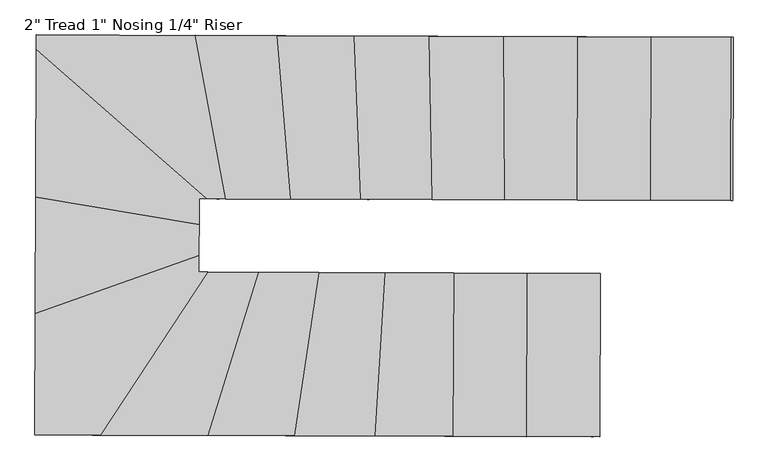
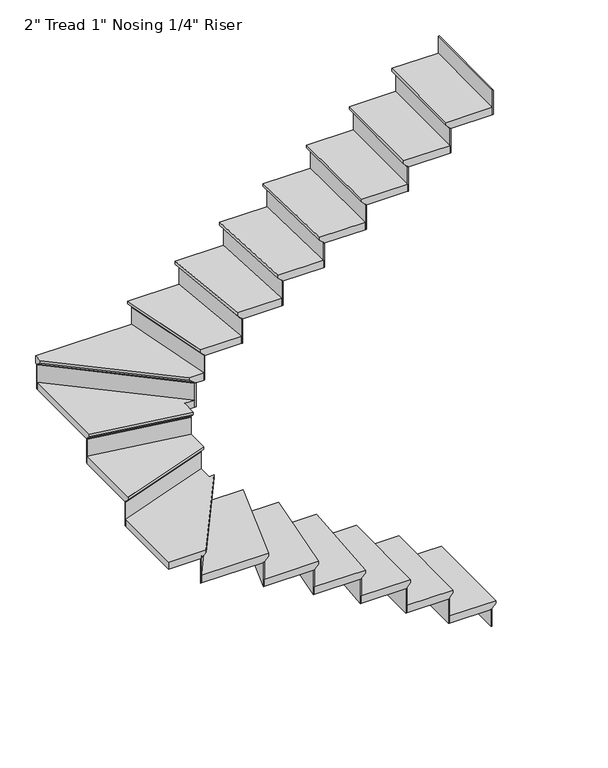
"""IFC4 building model written with IfcOpenShell, lengths in millimetres: stair flight geometry."""

from ifc_helpers import new_model, si_unit, origin, place, context, project, spatial, faceted_brep, source, transform, mapped, element, save


def stair_flight_f5e35143(model_context):
    return source(origin(), model_context, "Body", "Brep", [
        faceted_brep([(-2339.9228929, -4204.0248458, 6551.0833333), (-2339.9228929, -4204.0248458, 6570.1333333), (-2342.0274141, -4826.0015756, 6570.1333333), (-2342.0274141, -4826.0015756, 6551.0833333), (-2365.3227475, -4203.9389029, 6525.6833333), (-2367.4272687, -4825.9156326, 6525.6833333), (-2644.7211481, -4202.9935301, 6570.1333333), (-2646.8256693, -4824.9702599, 6570.1333333), (-2367.4272687, -4825.9156326, 6519.3333333), (-2646.8256693, -4824.9702599, 6519.3333333), (-2644.7211481, -4202.9935301, 6519.3333333), (-2365.3227475, -4203.9389029, 6519.3333333)], [[[0, 1, 2, 3]], [[4, 0, 3, 5]], [[2, 1, 6, 7]], [[8, 9, 10, 11]], [[2, 7, 9, 8, 5, 3]], [[8, 11, 4, 5]], [[6, 1, 0, 4, 11, 10]], [[7, 6, 10, 9]]]),
        faceted_brep([(-2365.3227475, -4203.9389029, 6519.3333333), (-2365.3227475, -4203.9389029, 6400.8), (-2371.6727112, -4203.9174171, 6400.8), (-2371.6727112, -4203.9174171, 6519.3333333), (-2367.4272687, -4825.9156326, 6519.3333333), (-2373.7772323, -4825.8941469, 6519.3333333), (-2373.7772323, -4825.8941469, 6400.8), (-2367.4272687, -4825.9156326, 6400.8)], [[[0, 1, 2, 3]], [[4, 5, 6, 7]], [[1, 0, 4, 7]], [[2, 1, 7, 6]], [[3, 2, 6, 5]], [[0, 3, 5, 4]]]),
        faceted_brep([(-2644.7211481, -4202.9935301, 6688.6666667), (-2644.7211481, -4202.9935301, 6519.3333333), (-2651.0711118, -4202.9720444, 6519.3333333), (-2651.0711118, -4202.9720444, 6688.6666667), (-2646.8256693, -4824.9702599, 6688.6666667), (-2653.175633, -4824.9487741, 6688.6666667), (-2653.175633, -4824.9487741, 6519.3333333), (-2646.8256693, -4824.9702599, 6519.3333333)], [[[0, 1, 2, 3]], [[4, 5, 6, 7]], [[1, 0, 4, 7]], [[2, 1, 7, 6]], [[3, 2, 6, 5]], [[0, 3, 5, 4]]]),
        faceted_brep([(-2621.4258147, -4825.0562028, 6739.4666667), (-2619.3212935, -4203.0794731, 6739.4666667), (-2924.1195488, -4202.0481574, 6739.4666667), (-2926.2240699, -4824.0248871, 6739.4666667), (-2646.8256693, -4824.9702599, 6688.6666667), (-2926.2240699, -4824.0248871, 6688.6666667), (-2924.1195488, -4202.0481574, 6688.6666667), (-2644.7211481, -4202.9935301, 6688.6666667), (-2646.8256693, -4824.9702599, 6695.0166667), (-2621.4258147, -4825.0562028, 6720.4166667), (-2644.7211481, -4202.9935301, 6695.0166667), (-2619.3212935, -4203.0794731, 6720.4166667)], [[[0, 1, 2, 3]], [[4, 5, 6, 7]], [[0, 3, 5, 4, 8, 9]], [[4, 7, 10, 8]], [[2, 1, 11, 10, 7, 6]], [[3, 2, 6, 5]], [[11, 1, 0, 9]], [[10, 11, 9, 8]]]),
        faceted_brep([(-2924.1195488, -4202.0481574, 6858.0), (-2924.1195488, -4202.0481574, 6688.6666667), (-2930.4695124, -4202.0266716, 6688.6666667), (-2930.4695124, -4202.0266716, 6858.0), (-2926.2240699, -4824.0248871, 6858.0), (-2932.5740336, -4824.0034014, 6858.0), (-2932.5740336, -4824.0034014, 6688.6666667), (-2926.2240699, -4824.0248871, 6688.6666667)], [[[0, 1, 2, 3]], [[4, 5, 6, 7]], [[1, 0, 4, 7]], [[2, 1, 7, 6]], [[3, 2, 6, 5]], [[0, 3, 5, 4]]]),
        faceted_brep([(-2900.8242153, -4824.1108301, 6908.8), (-2898.7196941, -4202.1341003, 6908.8), (-3185.4282049, -4201.1639931, 6908.8), (-3223.7984946, -4823.0180139, 6908.8), (-2926.2240699, -4824.0248871, 6858.0), (-3223.7984946, -4823.0180139, 6858.0), (-3185.4282049, -4201.1639931, 6858.0), (-2924.1195488, -4202.0481574, 6858.0), (-2926.2240699, -4824.0248871, 6864.35), (-2900.8242153, -4824.1108301, 6889.75), (-2924.1195488, -4202.0481574, 6864.35), (-2898.7196941, -4202.1341003, 6889.75)], [[[0, 1, 2, 3]], [[4, 5, 6, 7]], [[0, 3, 5, 4, 8, 9]], [[4, 7, 10, 8]], [[2, 1, 11, 10, 7, 6]], [[3, 2, 6, 5]], [[11, 1, 0, 9]], [[10, 11, 9, 8]]]),
        faceted_brep([(-3185.4282049, -4201.1639931, 7027.3333333), (-3185.4282049, -4201.1639931, 6858.0), (-3191.7889535, -4201.1424708, 6858.0), (-3191.7889535, -4201.1424708, 7027.3333333), (-3223.7984946, -4823.0180139, 7027.3333333), (-3230.1592432, -4822.9964917, 7027.3333333), (-3230.1592432, -4822.9964917, 6858.0), (-3223.7984946, -4823.0180139, 6858.0)], [[[0, 1, 2, 3]], [[4, 5, 6, 7]], [[1, 0, 4, 7]], [[2, 1, 7, 6]], [[3, 2, 6, 5]], [[0, 3, 5, 4]]]),
        faceted_brep([(-3198.3555003, -4823.1041029, 7078.1333333), (-3159.9852105, -4201.250082, 7078.1333333), (-3437.1491731, -4200.3122697, 7078.1333333), (-3531.3418182, -4821.97741, 7078.1333333), (-3223.7984946, -4823.0180139, 7027.3333333), (-3531.3418182, -4821.97741, 7027.3333333), (-3437.1491731, -4200.3122697, 7027.3333333), (-3185.4282049, -4201.1639931, 7027.3333333), (-3223.7984946, -4823.0180139, 7033.6833333), (-3198.3555003, -4823.1041029, 7059.0833333), (-3185.4282049, -4201.1639931, 7033.6833333), (-3159.9852105, -4201.250082, 7059.0833333)], [[[0, 1, 2, 3]], [[4, 5, 6, 7]], [[0, 3, 5, 4, 8, 9]], [[4, 7, 10, 8]], [[2, 1, 11, 10, 7, 6]], [[3, 2, 6, 5]], [[11, 1, 0, 9]], [[10, 11, 9, 8]]]),
        faceted_brep([(-3437.1491731, -4200.3122697, 7196.6666667), (-3437.1491731, -4200.3122697, 7027.3333333), (-3443.568358, -4200.2905498, 7027.3333333), (-3443.568358, -4200.2905498, 7196.6666667), (-3531.3418182, -4821.97741, 7196.6666667), (-3537.7610031, -4821.95569, 7196.6666667), (-3537.7610031, -4821.95569, 7027.3333333), (-3531.3418182, -4821.97741, 7027.3333333)], [[[0, 1, 2, 3]], [[4, 5, 6, 7]], [[1, 0, 4, 7]], [[2, 1, 7, 6]], [[3, 2, 6, 5]], [[0, 3, 5, 4]]]),
        faceted_brep([(-3505.6650785, -4822.0642898, 7247.4666667), (-3411.4724335, -4200.3991496, 7247.4666667), (-3668.9000376, -4199.5281172, 7247.4666667), (-3860.1305452, -4820.8649201, 7247.4666667), (-3531.3418182, -4821.97741, 7196.6666667), (-3860.1305452, -4820.8649201, 7196.6666667), (-3668.9000376, -4199.5281172, 7196.6666667), (-3437.1491731, -4200.3122697, 7196.6666667), (-3531.3418182, -4821.97741, 7203.0166667), (-3505.6650785, -4822.0642898, 7228.4166667), (-3437.1491731, -4200.3122697, 7203.0166667), (-3411.4724335, -4200.3991496, 7228.4166667)], [[[0, 1, 2, 3]], [[4, 5, 6, 7]], [[0, 3, 5, 4, 8, 9]], [[4, 7, 10, 8]], [[2, 1, 11, 10, 7, 6]], [[3, 2, 6, 5]], [[11, 1, 0, 9]], [[10, 11, 9, 8]]]),
        faceted_brep([(-3668.9000376, -4199.5281172, 7366.0), (-3668.9000376, -4199.5281172, 7196.6666667), (-3675.5370713, -4199.5056601, 7196.6666667), (-3675.5370713, -4199.5056601, 7366.0), (-3860.1305452, -4820.8649201, 7366.0), (-3866.7675788, -4820.842463, 7366.0), (-3866.7675788, -4820.842463, 7196.6666667), (-3860.1305452, -4820.8649201, 7196.6666667)], [[[0, 1, 2, 3]], [[4, 5, 6, 7]], [[1, 0, 4, 7]], [[2, 1, 7, 6]], [[3, 2, 6, 5]], [[0, 3, 5, 4]]]),
        faceted_brep([(-3833.5824104, -4820.9547484, 7416.8), (-3642.3519028, -4199.6179455, 7416.8), (-3864.4957991, -4198.8662992, 7416.8), (-4274.0422035, -4819.4644081, 7416.8), (-3860.1305452, -4820.8649201, 7366.0), (-4274.0422035, -4819.4644081, 7366.0), (-3864.4957991, -4198.8662992, 7366.0), (-3668.9000376, -4199.5281172, 7366.0), (-3860.1305452, -4820.8649201, 7372.35), (-3833.5824104, -4820.9547484, 7397.75), (-3668.9000376, -4199.5281172, 7372.35), (-3642.3519028, -4199.6179455, 7397.75)], [[[0, 1, 2, 3]], [[4, 5, 6, 7]], [[0, 3, 5, 4, 8, 9]], [[4, 7, 10, 8]], [[2, 1, 11, 10, 7, 6]], [[3, 2, 6, 5]], [[11, 1, 0, 9]], [[10, 11, 9, 8]]]),
        faceted_brep([(-3864.4957991, -4198.8662992, 7535.3333333), (-3864.4957991, -4198.8662992, 7366.0), (-3872.0869257, -4198.8406138, 7366.0), (-3872.0869257, -4198.8406138, 7535.3333333), (-4274.0422035, -4819.4644081, 7535.3333333), (-4281.6333301, -4819.4387227, 7535.3333333), (-4281.6333301, -4819.4387227, 7366.0), (-4274.0422035, -4819.4644081, 7366.0)], [[[0, 1, 2, 3]], [[4, 5, 6, 7]], [[1, 0, 4, 7]], [[2, 1, 7, 6]], [[3, 2, 6, 5]], [[0, 3, 5, 4]]]),
        faceted_brep([(-4490.0684734, -4328.5349965, 7586.1333333), (-4491.7270905, -4818.7278493, 7586.1333333), (-4243.677697, -4819.5671495, 7586.1333333), (-3834.1312926, -4198.9690405, 7586.1333333), (-3867.6458395, -4198.8556407, 7586.1333333), (-3867.338948, -4108.1559559, 7586.1333333), (-4491.7270905, -4818.7278493, 7535.3333333), (-4490.0684734, -4328.5349965, 7535.3333333), (-3867.338948, -4108.1559559, 7535.3333333), (-3867.6458395, -4198.8556407, 7535.3333333), (-3864.4957991, -4198.8662992, 7535.3333333), (-4274.0422035, -4819.4644081, 7535.3333333), (-4274.0422035, -4819.4644081, 7541.6833333), (-4243.677697, -4819.5671495, 7567.0833333), (-3864.4957991, -4198.8662992, 7541.6833333), (-3834.1312926, -4198.9690405, 7567.0833333)], [[[0, 1, 2, 3, 4, 5]], [[6, 7, 8, 9, 10, 11]], [[1, 0, 7, 6]], [[2, 1, 6, 11, 12, 13]], [[11, 10, 14, 12]], [[4, 3, 15, 14, 10, 9]], [[5, 4, 9, 8]], [[0, 5, 8, 7]], [[15, 3, 2, 13]], [[14, 15, 13, 12]]]),
        faceted_brep([(-3867.338948, -4108.1559559, 7704.6666667), (-3867.338948, -4108.1559559, 7535.3333333), (-3867.316129, -4101.4119712, 7535.3333333), (-3867.316129, -4101.4119712, 7704.6666667), (-4490.0684734, -4328.5349965, 7704.6666667), (-4490.0456544, -4321.7910118, 7704.6666667), (-4490.0456544, -4321.7910118, 7535.3333333), (-4490.0684734, -4328.5349965, 7535.3333333)], [[[0, 1, 2, 3]], [[4, 5, 6, 7]], [[1, 0, 4, 7]], [[2, 1, 7, 6]], [[3, 2, 6, 5]], [[0, 3, 5, 4]]]),
        faceted_brep([(-4490.1597492, -4355.5109354, 7755.4666667), (-3867.4302238, -4135.1318948, 7755.4666667), (-3866.9449143, -3991.702012, 7755.4666667), (-4488.5718319, -3886.2129338, 7755.4666667), (-4490.0684734, -4328.5349965, 7704.6666667), (-4488.5718319, -3886.2129338, 7704.6666667), (-3866.9449143, -3991.702012, 7704.6666667), (-3867.338948, -4108.1559559, 7704.6666667), (-4490.0684734, -4328.5349965, 7711.0166667), (-4490.1597492, -4355.5109354, 7736.4166667), (-3867.338948, -4108.1559559, 7711.0166667), (-3867.4302238, -4135.1318948, 7736.4166667)], [[[0, 1, 2, 3]], [[4, 5, 6, 7]], [[0, 3, 5, 4, 8, 9]], [[4, 7, 10, 8]], [[3, 2, 6, 5]], [[11, 1, 0, 9]], [[10, 11, 9, 8]], [[2, 1, 11, 10, 7, 6]]]),
        faceted_brep([(-3866.9449143, -3991.702012, 7874.0), (-3866.9449143, -3991.702012, 7704.6666667), (-3866.9231337, -3985.2649249, 7704.6666667), (-3866.9231337, -3985.2649249, 7874.0), (-4488.5718319, -3886.2129338, 7874.0), (-4488.5500514, -3879.7758467, 7874.0), (-4488.5500514, -3879.7758467, 7704.6666667), (-4488.5718319, -3886.2129338, 7704.6666667)], [[[0, 1, 2, 3]], [[4, 5, 6, 7]], [[1, 0, 4, 7]], [[2, 1, 7, 6]], [[3, 2, 6, 5]], [[0, 3, 5, 4]]]),
        faceted_brep([(-4488.6589541, -3911.9612823, 7924.8), (-3867.0320364, -4017.4503605, 7924.8), (-3866.7004668, -3919.4572401, 7924.8), (-3799.1127501, -3919.6859299, 7924.8), (-4486.6423896, -3315.9795656, 7924.8), (-4488.5718319, -3886.2129338, 7874.0), (-4486.6423896, -3315.9795656, 7874.0), (-3799.1127501, -3919.6859299, 7874.0), (-3866.7004668, -3919.4572401, 7874.0), (-3866.9449143, -3991.702012, 7874.0), (-4488.5718319, -3886.2129338, 7880.35), (-4488.6589541, -3911.9612823, 7905.75), (-3866.9449143, -3991.702012, 7880.35), (-3867.0320364, -4017.4503605, 7905.75)], [[[0, 1, 2, 3, 4]], [[5, 6, 7, 8, 9]], [[0, 4, 6, 5, 10, 11]], [[5, 9, 12, 10]], [[2, 1, 13, 12, 9, 8]], [[4, 3, 7, 6]], [[13, 1, 0, 11]], [[12, 13, 11, 10]], [[3, 2, 8, 7]]]),
        faceted_brep([(-3799.1127501, -3919.6859299, 8043.3333333), (-3799.1127501, -3919.6859299, 7874.0), (-3789.4516067, -3919.7186194, 7874.0), (-3789.4516067, -3919.7186194, 8043.3333333), (-4486.6423896, -3315.9795656, 8043.3333333), (-4486.613881, -3307.5540264, 8043.3333333), (-4486.613881, -3307.5540264, 7874.0), (-4486.6423896, -3315.9795656, 7874.0)], [[[0, 1, 2, 3]], [[4, 5, 6, 7]], [[1, 0, 4, 7]], [[2, 1, 7, 6]], [[3, 2, 6, 5]], [[0, 3, 5, 4]]]),
        faceted_brep([(-3855.3688773, -3297.511731, 8094.1333333), (-4486.5726753, -3295.3759891, 8094.1333333), (-4486.7564243, -3349.6817226, 8094.1333333), (-3837.757324, -3919.5551721, 8094.1333333), (-3739.9081193, -3919.8862548, 8094.1333333), (-4486.5726753, -3295.3759891, 8043.3333333), (-3855.3688773, -3297.511731, 8043.3333333), (-3739.9081193, -3919.8862548, 8043.3333333), (-3799.1127501, -3919.6859299, 8043.3333333), (-4486.6423896, -3315.9795656, 8043.3333333), (-3799.1127501, -3919.6859299, 8049.6833333), (-4486.6423896, -3315.9795656, 8049.6833333), (-3837.757324, -3919.5551721, 8075.0833333), (-4486.7564243, -3349.6817226, 8075.0833333)], [[[0, 1, 2, 3, 4]], [[5, 6, 7, 8, 9]], [[1, 0, 6, 5]], [[9, 8, 10, 11]], [[4, 3, 12, 10, 8, 7]], [[0, 4, 7, 6]], [[12, 3, 2, 13]], [[10, 12, 13, 11]], [[2, 1, 5, 9, 11, 13]]]),
        faceted_brep([(-3739.9081193, -3919.8862548, 8212.6666667), (-3739.9081193, -3919.8862548, 8043.3333333), (-3733.4457151, -3919.908121, 8043.3333333), (-3733.4457151, -3919.908121, 8212.6666667), (-3855.3688773, -3297.511731, 8212.6666667), (-3848.9064731, -3297.5335972, 8212.6666667), (-3848.9064731, -3297.5335972, 8043.3333333), (-3855.3688773, -3297.511731, 8043.3333333)], [[[0, 1, 2, 3]], [[4, 5, 6, 7]], [[1, 0, 4, 7]], [[2, 1, 7, 6]], [[3, 2, 6, 5]], [[0, 3, 5, 4]]]),
        faceted_brep([(-3881.2184941, -3297.4242662, 8263.4666667), (-3765.7577361, -3919.79879, 8263.4666667), (-3493.4024921, -3920.7203315, 8263.4666667), (-3543.7965904, -3298.5659674, 8263.4666667), (-3855.3688773, -3297.511731, 8212.6666667), (-3543.7965904, -3298.5659674, 8212.6666667), (-3493.4024921, -3920.7203315, 8212.6666667), (-3739.9081193, -3919.8862548, 8212.6666667), (-3855.3688773, -3297.511731, 8219.0166667), (-3881.2184941, -3297.4242662, 8244.4166667), (-3739.9081193, -3919.8862548, 8219.0166667), (-3765.7577361, -3919.79879, 8244.4166667)], [[[0, 1, 2, 3]], [[4, 5, 6, 7]], [[0, 3, 5, 4, 8, 9]], [[4, 7, 10, 8]], [[2, 1, 11, 10, 7, 6]], [[3, 2, 6, 5]], [[11, 1, 0, 9]], [[10, 11, 9, 8]]]),
        faceted_brep([(-3493.4024921, -3920.7203315, 8382.0), (-3493.4024921, -3920.7203315, 8212.6666667), (-3487.0299488, -3920.7418937, 8212.6666667), (-3487.0299488, -3920.7418937, 8382.0), (-3543.7965904, -3298.5659674, 8382.0), (-3537.4240471, -3298.5875295, 8382.0), (-3537.4240471, -3298.5875295, 8212.6666667), (-3543.7965904, -3298.5659674, 8212.6666667)], [[[0, 1, 2, 3]], [[4, 5, 6, 7]], [[1, 0, 4, 7]], [[2, 1, 7, 6]], [[3, 2, 6, 5]], [[0, 3, 5, 4]]]),
        faceted_brep([(-3569.2867636, -3298.4797188, 8432.8), (-3518.8926653, -3920.634083, 8432.8), (-3226.664936, -3921.622865, 8432.8), (-3251.8690415, -3299.5537338, 8432.8), (-3543.7965904, -3298.5659674, 8382.0), (-3251.8690415, -3299.5537338, 8382.0), (-3226.664936, -3921.622865, 8382.0), (-3493.4024921, -3920.7203315, 8382.0), (-3543.7965904, -3298.5659674, 8388.35), (-3569.2867636, -3298.4797188, 8413.75), (-3493.4024921, -3920.7203315, 8388.35), (-3518.8926653, -3920.634083, 8413.75)], [[[0, 1, 2, 3]], [[4, 5, 6, 7]], [[0, 3, 5, 4, 8, 9]], [[4, 7, 10, 8]], [[2, 1, 11, 10, 7, 6]], [[3, 2, 6, 5]], [[11, 1, 0, 9]], [[10, 11, 9, 8]]]),
        faceted_brep([(-3226.664936, -3921.622865, 8551.3333333), (-3226.664936, -3921.622865, 8382.0), (-3220.3088547, -3921.6443715, 8382.0), (-3220.3088547, -3921.6443715, 8551.3333333), (-3251.8690415, -3299.5537338, 8551.3333333), (-3245.5129602, -3299.5752402, 8551.3333333), (-3245.5129602, -3299.5752402, 8382.0), (-3251.8690415, -3299.5537338, 8382.0)], [[[0, 1, 2, 3]], [[4, 5, 6, 7]], [[1, 0, 4, 7]], [[2, 1, 7, 6]], [[3, 2, 6, 5]], [[0, 3, 5, 4]]]),
        faceted_brep([(-3277.2933666, -3299.467708, 8602.1333333), (-3252.0892611, -3921.5368393, 8602.1333333), (-2953.9711928, -3922.5455519, 8602.1333333), (-2965.8021755, -3300.52167, 8602.1333333), (-3251.8690415, -3299.5537338, 8551.3333333), (-2965.8021755, -3300.52167, 8551.3333333), (-2953.9711928, -3922.5455519, 8551.3333333), (-3226.664936, -3921.622865, 8551.3333333), (-3251.8690415, -3299.5537338, 8557.6833333), (-3277.2933666, -3299.467708, 8583.0833333), (-3226.664936, -3921.622865, 8557.6833333), (-3252.0892611, -3921.5368393, 8583.0833333)], [[[0, 1, 2, 3]], [[4, 5, 6, 7]], [[0, 3, 5, 4, 8, 9]], [[4, 7, 10, 8]], [[2, 1, 11, 10, 7, 6]], [[3, 2, 6, 5]], [[11, 1, 0, 9]], [[10, 11, 9, 8]]]),
        faceted_brep([(-2953.9711928, -3922.5455519, 8720.6666667), (-2953.9711928, -3922.5455519, 8551.3333333), (-2947.6196355, -3922.567043, 8551.3333333), (-2947.6196355, -3922.567043, 8720.6666667), (-2965.8021755, -3300.52167, 8720.6666667), (-2959.4506182, -3300.5431611, 8720.6666667), (-2959.4506182, -3300.5431611, 8551.3333333), (-2965.8021755, -3300.52167, 8551.3333333)], [[[0, 1, 2, 3]], [[4, 5, 6, 7]], [[1, 0, 4, 7]], [[2, 1, 7, 6]], [[3, 2, 6, 5]], [[0, 3, 5, 4]]]),
        faceted_brep([(-2991.2084046, -3300.4357054, 8771.4666667), (-2979.3774219, -3922.4595874, 8771.4666667), (-2678.7239035, -3923.476879, 8771.4666667), (-2682.2633211, -3301.4810524, 8771.4666667), (-2965.8021755, -3300.52167, 8720.6666667), (-2682.2633211, -3301.4810524, 8720.6666667), (-2678.7239035, -3923.476879, 8720.6666667), (-2953.9711928, -3922.5455519, 8720.6666667), (-2965.8021755, -3300.52167, 8727.0166667), (-2991.2084046, -3300.4357054, 8752.4166667), (-2953.9711928, -3922.5455519, 8727.0166667), (-2979.3774219, -3922.4595874, 8752.4166667)], [[[0, 1, 2, 3]], [[4, 5, 6, 7]], [[0, 3, 5, 4, 8, 9]], [[4, 7, 10, 8]], [[2, 1, 11, 10, 7, 6]], [[3, 2, 6, 5]], [[11, 1, 0, 9]], [[10, 11, 9, 8]]]),
        faceted_brep([(-2678.7239035, -3923.476879, 8890.0), (-2678.7239035, -3923.476879, 8720.6666667), (-2672.3736784, -3923.4983656, 8720.6666667), (-2672.3736784, -3923.4983656, 8890.0), (-2682.2633211, -3301.4810524, 8890.0), (-2675.913096, -3301.502539, 8890.0), (-2675.913096, -3301.502539, 8720.6666667), (-2682.2633211, -3301.4810524, 8720.6666667)], [[[0, 1, 2, 3]], [[4, 5, 6, 7]], [[1, 0, 4, 7]], [[2, 1, 7, 6]], [[3, 2, 6, 5]], [[0, 3, 5, 4]]]),
        faceted_brep([(-2707.6642214, -3301.3951058, 8940.8), (-2704.1248038, -3923.3909324, 8940.8), (-2402.148518, -3924.4126998, 8940.8), (-2400.0439968, -3302.43597, 8940.8), (-2682.2633211, -3301.4810524, 8890.0), (-2400.0439968, -3302.43597, 8890.0), (-2402.148518, -3924.4126998, 8890.0), (-2678.7239035, -3923.476879, 8890.0), (-2682.2633211, -3301.4810524, 8896.35), (-2707.6642214, -3301.3951058, 8921.75), (-2678.7239035, -3923.476879, 8896.35), (-2704.1248038, -3923.3909324, 8921.75)], [[[0, 1, 2, 3]], [[4, 5, 6, 7]], [[0, 3, 5, 4, 8, 9]], [[4, 7, 10, 8]], [[2, 1, 11, 10, 7, 6]], [[3, 2, 6, 5]], [[11, 1, 0, 9]], [[10, 11, 9, 8]]]),
        faceted_brep([(-2402.148518, -3924.4126998, 9059.3333333), (-2402.148518, -3924.4126998, 8890.0), (-2395.7985543, -3924.4341855, 8890.0), (-2395.7985543, -3924.4341855, 9059.3333333), (-2400.0439968, -3302.43597, 9059.3333333), (-2393.6940331, -3302.4574557, 9059.3333333), (-2393.6940331, -3302.4574557, 8890.0), (-2400.0439968, -3302.43597, 8890.0)], [[[0, 1, 2, 3]], [[4, 5, 6, 7]], [[1, 0, 4, 7]], [[2, 1, 7, 6]], [[3, 2, 6, 5]], [[0, 3, 5, 4]]]),
        faceted_brep([(-2425.4438514, -3302.350027, 9110.1333333), (-2427.5483726, -3924.3267568, 9110.1333333), (-2122.7501174, -3925.3580725, 9110.1333333), (-2120.6455962, -3303.3813428, 9110.1333333), (-2400.0439968, -3302.43597, 9059.3333333), (-2120.6455962, -3303.3813428, 9059.3333333), (-2122.7501174, -3925.3580725, 9059.3333333), (-2402.148518, -3924.4126998, 9059.3333333), (-2400.0439968, -3302.43597, 9065.6833333), (-2425.4438514, -3302.350027, 9091.0833333), (-2402.148518, -3924.4126998, 9065.6833333), (-2427.5483726, -3924.3267568, 9091.0833333)], [[[0, 1, 2, 3]], [[4, 5, 6, 7]], [[0, 3, 5, 4, 8, 9]], [[4, 7, 10, 8]], [[2, 1, 11, 10, 7, 6]], [[3, 2, 6, 5]], [[11, 1, 0, 9]], [[10, 11, 9, 8]]]),
        faceted_brep([(-2122.7501174, -3925.3580725, 9228.6666667), (-2122.7501174, -3925.3580725, 9059.3333333), (-2116.4001537, -3925.3795583, 9059.3333333), (-2116.4001537, -3925.3795583, 9228.6666667), (-2120.6455962, -3303.3813428, 9228.6666667), (-2114.2956325, -3303.4028285, 9228.6666667), (-2114.2956325, -3303.4028285, 9059.3333333), (-2120.6455962, -3303.3813428, 9059.3333333)], [[[0, 1, 2, 3]], [[4, 5, 6, 7]], [[1, 0, 4, 7]], [[2, 1, 7, 6]], [[3, 2, 6, 5]], [[0, 3, 5, 4]]]),
        faceted_brep([(-1843.3517167, -3926.3034453, 9398.0), (-1843.3517167, -3926.3034453, 9228.6666667), (-1837.0017531, -3926.324931, 9228.6666667), (-1837.0017531, -3926.324931, 9398.0), (-1841.2471955, -3304.3267155, 9398.0), (-1834.8972319, -3304.3482013, 9398.0), (-1834.8972319, -3304.3482013, 9228.6666667), (-1841.2471955, -3304.3267155, 9228.6666667)], [[[0, 1, 2, 3]], [[4, 5, 6, 7]], [[1, 0, 4, 7]], [[2, 1, 7, 6]], [[3, 2, 6, 5]], [[0, 3, 5, 4]]]),
        faceted_brep([(-2146.0454508, -3303.2953998, 9279.4666667), (-2148.149972, -3925.2721295, 9279.4666667), (-1843.3517167, -3926.3034453, 9279.4666667), (-1841.2471955, -3304.3267155, 9279.4666667), (-2120.6455962, -3303.3813428, 9228.6666667), (-1841.2471955, -3304.3267155, 9228.6666667), (-1843.3517167, -3926.3034453, 9228.6666667), (-2122.7501174, -3925.3580725, 9228.6666667), (-2120.6455962, -3303.3813428, 9235.0166667), (-2146.0454508, -3303.2953998, 9260.4166667), (-2122.7501174, -3925.3580725, 9235.0166667), (-2148.149972, -3925.2721295, 9260.4166667)], [[[0, 1, 2, 3]], [[4, 5, 6, 7]], [[0, 3, 5, 4, 8, 9]], [[4, 7, 10, 8]], [[2, 1, 11, 10, 7, 6]], [[3, 2, 6, 5]], [[11, 1, 0, 9]], [[10, 11, 9, 8]]]),
    ])


if __name__ == "__main__":
    model = new_model("IFC4")
    model_context = context("Model", 3, world=origin())
    ifc_project = project(units=[si_unit("LENGTHUNIT", "METRE", prefix="MILLI")], contexts=[model_context])
    site = spatial("IfcSite", under=ifc_project)
    building = spatial("IfcBuilding", under=site)
    placement = place(None, origin())
    stair_flight_shape = stair_flight_f5e35143(model_context)
    element("IfcStairFlight", 1, ObjectType="2\" Tread 1\" Nosing 1/4\" Riser", at=placement, inside=building, context=model_context, shape_type="MappedRepresentation", body=[
        mapped(stair_flight_shape, transform((0.0, 0.0, 0.0), x_axis=(1.0, 0.0, 0.0), y_axis=(0.0, 1.0, 0.0), z_axis=(0.0, 0.0, 1.0))),
    ])
    save(model, "model.ifc")
